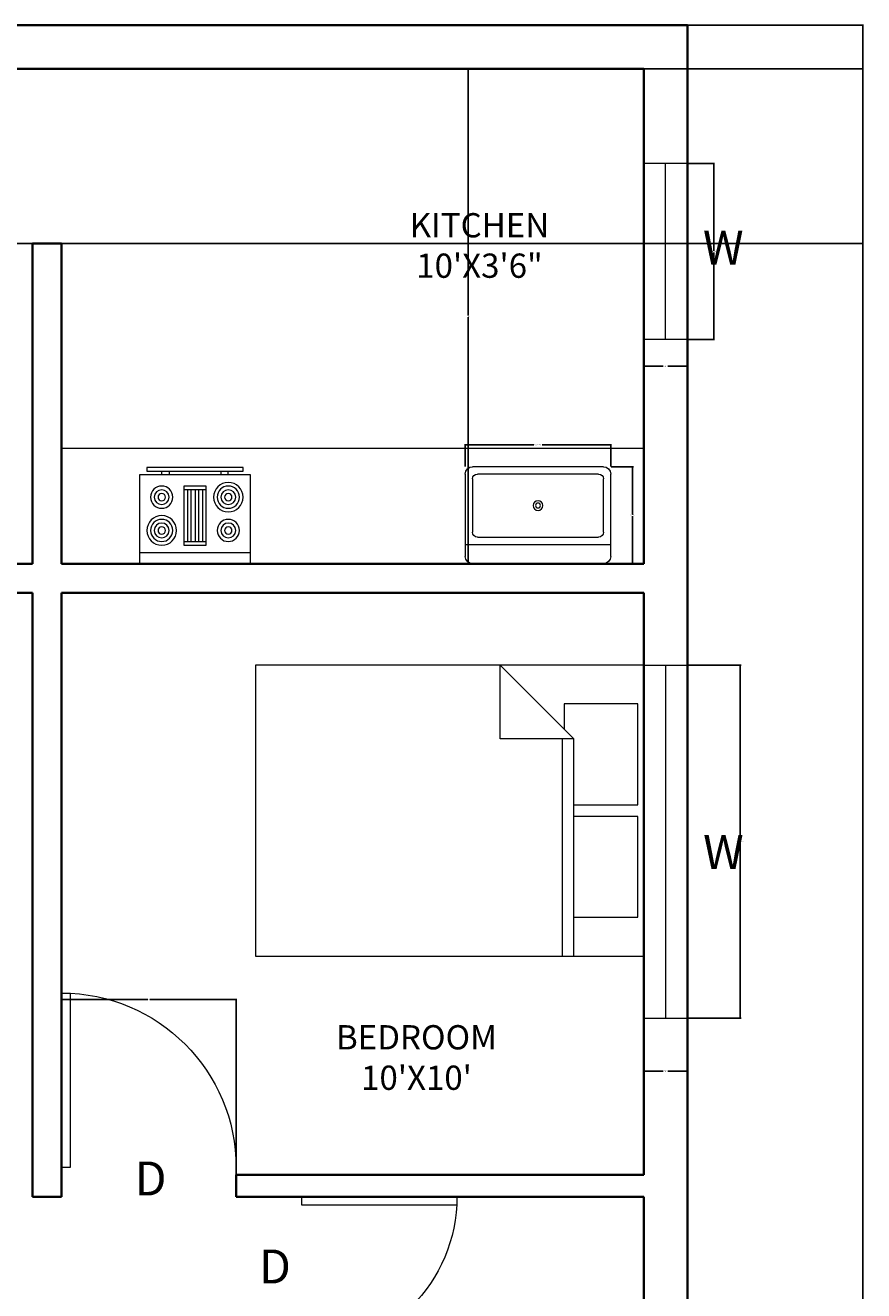
# Model space of a CAD drawing. Units: inches. Extents: x 1939 to 2674, y 558 to 1170.
# Tile 6 of 6: x 2502 to 2674, y 873 to 1134. Entities that reach past the tile are written whole.
import ezdxf

# ---------------------------------------------------------------- set-up
doc = ezdxf.new("R2010")
doc.units = ezdxf.units.IN
for name, color, linetype, lineweight in [('A-ANNO-DIMS', 2, 'Continuous', 18), ('A-ANNO-TEXT', 7, 'Continuous', 18), ('A-AREA-IDEN', 7, 'Continuous', 18), ('A-DOOR', 3, 'Continuous', 18), ('A-EQPM', 8, 'Continuous', 18), ('A-FLOR-CASE', 8, 'Continuous', 18), ('A-FLOR-FIXT', 9, 'Continuous', 18), ('A-FURN', 8, 'Continuous', 13), ('A-GLAZ', 4, 'Continuous', 18), ('A-WALL', 7, 'Continuous', 35)]:
    doc.layers.add(name, color=color, linetype=linetype, lineweight=lineweight)
doc.styles.get("Standard").update_dxf_attribs({"font": 'arial.ttf'})
doc.dimstyles.get("Standard").update_dxf_attribs({"dimtxt": 0.18, "dimasz": 0.18, "dimexe": 0.18, "dimexo": 0.0625, "dimgap": 0.09, "dimtad": 0, "dimtih": 1, "dimtoh": 1, "dimdec": 4, "dimzin": 0, "dimdsep": 46, "dimtxsty": 'Standard', "dimcen": 0.09, "dimadec": 0, "dimazin": 0, "dimtfac": 1, "dimtdec": 4, "dimtofl": 0, "dimtmove": 0, "dimatfit": 3, "dimfxl": 1, "dimtolj": 1, "dimtzin": 0, "dimarcsym": 0})

# ---------------------------------------------------------------- blocks, each defined once
blk = doc.blocks.new('Bed - Queen')
for p, q in [((0, -80.00003), (0, 0)), ((0, 0), (59.99999, 0)), ((59.99999, 0), (59.99999, -80.00003)), ((7.99999, -1.2), (28.79998, -1.2)), ((7.99999, -14.4), (7.99999, -1.2)), ((28.79998, -1.2), (28.79998, -14.4)), ((31.19999, -1.2), (51.99999, -1.2)), ((31.19999, -14.4), (31.19999, -1.2)), ((51.99999, -1.2), (51.99999, -16.4)), ((0, -14.4), (44.8, -14.4)), ((59.99999, -29.6), (44.8, -14.4)), ((44.8, -14.4), (44.8, -29.6)), ((44.8, -16.8), (0, -16.8)), ((51.99999, -16.4), (46.79936, -16.4)), ((44.8, -29.6), (59.99999, -29.6)), ((59.99999, -80.00003), (0, -80.00003))]:
    blk.add_line(p, q)
blk = doc.blocks.new('Sink-single - 30 in top')
blk.add_line((-15, -3.999996), (15, -3.999996))
for points in [[(-13.5, 0), (13.5, 0)], [(-15, -18.499996), (-15, -1.5)], [(15, -1.5), (15, -18.499996)], [(-13.5, -17.499996), (-13.5, -6.499996)], [(-12.5, -5.499996), (12.5, -5.499996)], [(13.5, -6.499996), (13.5, -17.499996)], [(13.5, -19.999996), (-13.5, -19.999996)], [(12.5, -18.499996), (-12.5, -18.499996)]]:
    blk.add_lwpolyline(points)
for radius in [1, 0.5]:
    blk.add_circle((0, -11.999996), radius)
for centre, radius, start, end in [((-13.5, -1.5), 1.5, 90, 180), ((13.5, -1.5), 1.5, 0, 90), ((-12.5, -6.499996), 1, 90, 180), ((12.5, -6.499996), 1, 0, 90), ((-12.5, -17.499996), 1, 180, 270), ((12.5, -17.499996), 1, 270, 0), ((-13.5, -18.499996), 1.5, 180, 270), ((13.5, -18.499996), 1.5, 270, 0)]:
    blk.add_arc(centre, radius, start, end)
blk = doc.blocks.new('Range-Oven - 30 in top')
for p, q in [((0, -3), (30, -3)), ((12, -6), (18, -6)), ((13, -20), (13, -6)), ((14, -6), (14, -20)), ((15, -20), (15, -6)), ((16, -6), (16, -20)), ((17, -20), (17, -6)), ((18, -20), (12, -20)), ((6, -24), (6, -25)), ((8, -25), (8, -24)), ((22, -25), (22, -24)), ((24, -24), (24, -25))]:
    blk.add_line(p, q)
for points in [[(0, -24), (0, 0), (30, 0), (30, -24)], [(12, -21), (12, -5), (18, -5), (18, -21)], [(2, -26), (2, -25), (28, -25), (28, -26)]]:
    blk.add_lwpolyline(points, close=True)
for centre, radius in [((6, -9), 4), ((6, -9), 3), ((24, -9), 3), ((6, -9), 2), ((6, -9), 1), ((24, -9), 2), ((24, -9), 1), ((6, -18), 3), ((6, -18), 2), ((6, -18), 1), ((24, -18), 4), ((24, -18), 3), ((24, -18), 2), ((24, -18), 1)]:
    blk.add_circle(centre, radius)
blk = doc.blocks.new('*U10')
for p, q in [((0, 0), (0, -6)), ((-36, 0), (-36, -6))]:
    blk.add_line(p, q)
blk.add_lwpolyline([(0, 0), (0, 36), (-1.75, 36), (-1.75, 0)], close=True)
blk.add_arc((0, 0), 36, 90, 180)
blk = doc.blocks.new('*U12')
for p, q in [((0, 0), (0, -6)), ((-32, 0), (-32, -6))]:
    blk.add_line(p, q)
blk.add_lwpolyline([(0, 0), (0, 32), (-1.75, 32), (-1.75, 0)], close=True)
blk.add_arc((0, 0), 32, 90, 180)
blk = doc.blocks.new('WIN-KITCHEN')
for p, q in [((9, 36.3), (0, 36.3)), ((4.5, 0), (4.5, 36.3)), ((9, 0), (0, 0))]:
    blk.add_line(p, q)
blk = doc.blocks.new('WIN-BEDROOM')
for p, q in [((9, 72.81), (0, 72.81)), ((4.5, 0), (4.5, 72.81)), ((9, 0), (0, 0))]:
    blk.add_line(p, q)
blk = doc.blocks.new('*D30')
at = {"layer": 'A-ANNO-DIMS', "color": 0, "lineweight": -2, "transparency": 16777216}
for p, q in [((2592.27, 1043.17), (2592.27, 1047.79)), ((2592.45, 1047.61), (2606.41, 1047.61)), ((2622.09, 1047.61), (2608.12, 1047.61)), ((2622.27, 1043.17), (2622.27, 1047.79))]:
    blk.add_line(p, q, dxfattribs=at)
at = {"layer": 'A-ANNO-DIMS', "color": 0, "transparency": 16777216}
for points in [[(2592.45, 1047.64), (2592.45, 1047.58), (2592.27, 1047.61)], [(2622.09, 1047.64), (2622.09, 1047.58), (2622.27, 1047.61)]]:
    blk.add_solid(points, dxfattribs=at)
at = {"layer": 'Defpoints', "color": 0, "transparency": 16777216}
for p in [(2622.27, 1047.61), (2592.27, 1043.11), (2622.27, 1043.11)]:
    blk.add_point(p, dxfattribs=at)
at = {"layer": 'A-ANNO-DIMS', "color": 0, "transparency": 16777216, "insert": (2607.27, 1047.61), "char_height": 0.18, "attachment_point": 5}
blk.add_mtext('\\A1;SINK 30 TYP.', dxfattribs=at)
blk = doc.blocks.new('*D31')
at = {"layer": 'A-ANNO-DIMS', "color": 0, "lineweight": -2, "transparency": 16777216}
for p, q in [((2622.33, 1043.11), (2626.95, 1043.11)), ((2626.77, 1042.93), (2626.77, 1033.29)), ((2626.77, 1023.29), (2626.77, 1032.93)), ((2622.33, 1023.11), (2626.95, 1023.11))]:
    blk.add_line(p, q, dxfattribs=at)
at = {"layer": 'A-ANNO-DIMS', "color": 0, "transparency": 16777216}
for points in [[(2626.74, 1042.93), (2626.8, 1042.93), (2626.77, 1043.11)], [(2626.74, 1023.29), (2626.8, 1023.29), (2626.77, 1023.11)]]:
    blk.add_solid(points, dxfattribs=at)
at = {"layer": 'Defpoints', "color": 0, "transparency": 16777216}
for p in [(2622.27, 1043.11), (2622.27, 1023.11), (2626.77, 1023.11)]:
    blk.add_point(p, dxfattribs=at)
at = {"layer": 'A-ANNO-DIMS', "color": 0, "transparency": 16777216, "insert": (2626.77, 1033.11), "char_height": 0.18, "attachment_point": 5}
blk.add_mtext('\\A1;20 TYP.', dxfattribs=at)
blk = doc.blocks.new('*D40')
at = {"layer": 'A-ANNO-DIMS', "color": 0, "lineweight": -2, "transparency": 16777216}
for p, q in [((2638.11, 1105.6), (2643.67, 1105.6)), ((2643.49, 1105.42), (2643.49, 1087.64)), ((2643.49, 1069.49), (2643.49, 1087.27)), ((2638.11, 1069.31), (2643.67, 1069.31))]:
    blk.add_line(p, q, dxfattribs=at)
at = {"layer": 'A-ANNO-DIMS', "color": 0, "transparency": 16777216}
for points in [[(2643.46, 1105.42), (2643.52, 1105.42), (2643.49, 1105.6)], [(2643.46, 1069.49), (2643.52, 1069.49), (2643.49, 1069.31)]]:
    blk.add_solid(points, dxfattribs=at)
at = {"layer": 'Defpoints', "color": 0, "transparency": 16777216}
for p in [(2638.05, 1105.6), (2643.49, 1105.6), (2638.05, 1069.31)]:
    blk.add_point(p, dxfattribs=at)
at = {"layer": 'A-ANNO-DIMS', "color": 0, "transparency": 16777216, "insert": (2643.49, 1087.46), "char_height": 0.18, "attachment_point": 5}
blk.add_mtext('\\A1;WDW 36 TYP.', dxfattribs=at)
blk = doc.blocks.new('*D41')
at = {"layer": 'A-ANNO-DIMS', "color": 0, "lineweight": -2, "transparency": 16777216}
for p, q in [((2629.05, 1069.25), (2629.05, 1063.68)), ((2638.05, 1069.25), (2638.05, 1063.68)), ((2629.23, 1063.86), (2633.09, 1063.86)), ((2637.87, 1063.86), (2634.01, 1063.86))]:
    blk.add_line(p, q, dxfattribs=at)
at = {"layer": 'A-ANNO-DIMS', "color": 0, "transparency": 16777216}
for points in [[(2629.23, 1063.89), (2629.23, 1063.83), (2629.05, 1063.86)], [(2637.87, 1063.89), (2637.87, 1063.83), (2638.05, 1063.86)]]:
    blk.add_solid(points, dxfattribs=at)
at = {"layer": 'Defpoints', "color": 0, "transparency": 16777216}
for p in [(2629.05, 1069.31), (2638.05, 1069.31), (2638.05, 1063.86)]:
    blk.add_point(p, dxfattribs=at)
at = {"layer": 'A-ANNO-DIMS', "color": 0, "transparency": 16777216, "insert": (2633.55, 1063.86), "char_height": 0.18, "attachment_point": 5}
blk.add_mtext('\\A1;9 TYP.', dxfattribs=at)
blk = doc.blocks.new('*D42')
at = {"layer": 'A-ANNO-DIMS', "color": 0, "lineweight": -2, "transparency": 16777216}
for p, q in [((2638.11, 1002.22), (2649.15, 1002.22)), ((2648.97, 1002.04), (2648.97, 966)), ((2648.97, 929.59), (2648.97, 965.63)), ((2638.11, 929.41), (2649.15, 929.41))]:
    blk.add_line(p, q, dxfattribs=at)
at = {"layer": 'A-ANNO-DIMS', "color": 0, "transparency": 16777216}
for points in [[(2648.94, 1002.04), (2649, 1002.04), (2648.97, 1002.22)], [(2648.94, 929.59), (2649, 929.59), (2648.97, 929.41)]]:
    blk.add_solid(points, dxfattribs=at)
at = {"layer": 'Defpoints', "color": 0, "transparency": 16777216}
for p in [(2638.05, 1002.22), (2638.05, 929.41), (2648.97, 929.41)]:
    blk.add_point(p, dxfattribs=at)
at = {"layer": 'A-ANNO-DIMS', "color": 0, "transparency": 16777216, "insert": (2648.97, 965.82), "char_height": 0.18, "attachment_point": 5}
blk.add_mtext('\\A1;WDW 73 TYP.', dxfattribs=at)
blk = doc.blocks.new('*D43')
at = {"layer": 'A-ANNO-DIMS', "color": 0, "lineweight": -2, "transparency": 16777216}
for p, q in [((2629.05, 929.35), (2629.05, 918.31)), ((2638.05, 929.35), (2638.05, 918.31)), ((2629.23, 918.49), (2633.09, 918.49)), ((2637.87, 918.49), (2634.01, 918.49))]:
    blk.add_line(p, q, dxfattribs=at)
at = {"layer": 'A-ANNO-DIMS', "color": 0, "transparency": 16777216}
for points in [[(2629.23, 918.52), (2629.23, 918.46), (2629.05, 918.49)], [(2637.87, 918.52), (2637.87, 918.46), (2638.05, 918.49)]]:
    blk.add_solid(points, dxfattribs=at)
at = {"layer": 'Defpoints', "color": 0, "transparency": 16777216}
for p in [(2629.05, 929.41), (2638.05, 929.41), (2629.05, 918.49)]:
    blk.add_point(p, dxfattribs=at)
at = {"layer": 'A-ANNO-DIMS', "color": 0, "transparency": 16777216, "insert": (2633.55, 918.49), "char_height": 0.18, "attachment_point": 5}
blk.add_mtext('\\A1;9 TYP.', dxfattribs=at)
blk = doc.blocks.new('*D50')
at = {"layer": 'A-ANNO-DIMS', "color": 0, "lineweight": -2, "transparency": 16777216}
for p, q in [((2638.11, 1134.11), (2674.38, 1134.11)), ((2674.2, 1133.93), (2674.2, 864.29)), ((2674.2, 594.29), (2674.2, 863.93)), ((2638.11, 594.11), (2674.38, 594.11))]:
    blk.add_line(p, q, dxfattribs=at)
at = {"layer": 'A-ANNO-DIMS', "color": 0, "transparency": 16777216}
for points in [[(2674.17, 1133.93), (2674.23, 1133.93), (2674.2, 1134.11)], [(2674.17, 594.29), (2674.23, 594.29), (2674.2, 594.11)]]:
    blk.add_solid(points, dxfattribs=at)
at = {"layer": 'Defpoints', "color": 0, "transparency": 16777216}
for p in [(2638.05, 1134.11), (2674.2, 1134.11), (2638.05, 594.11)]:
    blk.add_point(p, dxfattribs=at)
at = {"layer": 'A-ANNO-DIMS', "color": 0, "transparency": 16777216, "insert": (2674.2, 864.11), "char_height": 0.18, "attachment_point": 5}
blk.add_mtext('\\A1;540', dxfattribs=at)
blk = doc.blocks.new('*D54')
at = {"layer": 'A-ANNO-DIMS', "color": 0, "lineweight": -2, "transparency": 16777216}
for p, q in [((2509.05, 897.17), (2509.05, 933.44)), ((2509.23, 933.26), (2526.83, 933.26)), ((2544.87, 933.26), (2527.27, 933.26)), ((2545.05, 897.17), (2545.05, 933.44))]:
    blk.add_line(p, q, dxfattribs=at)
at = {"layer": 'A-ANNO-DIMS', "color": 0, "transparency": 16777216}
for points in [[(2509.23, 933.29), (2509.23, 933.23), (2509.05, 933.26)], [(2544.87, 933.29), (2544.87, 933.23), (2545.05, 933.26)]]:
    blk.add_solid(points, dxfattribs=at)
at = {"layer": 'Defpoints', "color": 0, "transparency": 16777216}
for p in [(2545.05, 933.26), (2509.05, 897.11), (2545.05, 897.11)]:
    blk.add_point(p, dxfattribs=at)
at = {"layer": 'A-ANNO-DIMS', "color": 0, "transparency": 16777216, "insert": (2527.05, 933.26), "char_height": 0.18, "attachment_point": 5}
blk.add_mtext('\\A1;36', dxfattribs=at)
blk = doc.blocks.new('*D65')
at = {"layer": 'A-ANNO-DIMS', "color": 0, "lineweight": -2, "transparency": 16777216}
for p, q in [((2122.29, 1125.11), (2674.38, 1125.11)), ((2674.2, 1124.93), (2674.2, 1107.29)), ((2674.2, 1089.29), (2674.2, 1106.93)), ((2104.11, 1089.11), (2674.38, 1089.11))]:
    blk.add_line(p, q, dxfattribs=at)
at = {"layer": 'A-ANNO-DIMS', "color": 0, "transparency": 16777216}
for points in [[(2674.17, 1124.93), (2674.23, 1124.93), (2674.2, 1125.11)], [(2674.17, 1089.29), (2674.23, 1089.29), (2674.2, 1089.11)]]:
    blk.add_solid(points, dxfattribs=at)
at = {"layer": 'Defpoints', "color": 0, "transparency": 16777216}
for p in [(2122.22, 1125.11), (2674.2, 1125.11), (2104.05, 1089.11)]:
    blk.add_point(p, dxfattribs=at)
at = {"layer": 'A-ANNO-DIMS', "color": 0, "transparency": 16777216, "insert": (2674.2, 1107.11), "char_height": 0.18, "attachment_point": 5}
blk.add_mtext('\\A1;36', dxfattribs=at)
blk = doc.blocks.new('*D67')
at = {"layer": 'A-ANNO-DIMS', "color": 0, "lineweight": -2, "transparency": 16777216}
for p, q in [((2628.99, 1125.11), (2592.72, 1125.11)), ((2592.9, 1124.93), (2592.9, 1074.29)), ((2592.9, 1023.29), (2592.9, 1073.93)), ((2628.99, 1023.11), (2592.72, 1023.11))]:
    blk.add_line(p, q, dxfattribs=at)
at = {"layer": 'A-ANNO-DIMS', "color": 0, "transparency": 16777216}
for points in [[(2592.87, 1124.93), (2592.93, 1124.93), (2592.9, 1125.11)], [(2592.87, 1023.29), (2592.93, 1023.29), (2592.9, 1023.11)]]:
    blk.add_solid(points, dxfattribs=at)
at = {"layer": 'Defpoints', "color": 0, "transparency": 16777216}
for p in [(2592.9, 1125.11), (2629.05, 1125.11), (2629.05, 1023.11)]:
    blk.add_point(p, dxfattribs=at)
at = {"layer": 'A-ANNO-DIMS', "color": 0, "transparency": 16777216, "insert": (2592.9, 1074.11), "char_height": 0.18, "attachment_point": 5}
blk.add_mtext('\\A1;102', dxfattribs=at)

msp = doc.modelspace()

# ---------------------------------------------------------------- linework, layer by layer
at = {"layer": 'A-FLOR-CASE'}
msp.add_line((2629.048, 1046.8584), (2509.048, 1046.8584), dxfattribs=at)
at = {"layer": 'A-WALL'}
for p, q in [((2638.048, 1134.1102), (1975.048, 1134.1102)), ((2638.048, 594.1102), (2638.048, 1134.1102)), ((2638.048, 1134.1102), (2638.048, 594.1102)), ((2629.048, 1125.1102), (2383.048, 1125.1102)), ((2629.048, 1125.1102), (2629.048, 1023.1102)), ((2503.048, 1089.1102), (2503.048, 1023.1102)), ((2509.048, 1089.1102), (2503.048, 1089.1102)), ((2509.048, 1089.1102), (2509.048, 1023.1102)), ((2483.6519, 1023.1102), (2503.048, 1023.1102)), ((2509.048, 1023.1102), (2629.048, 1023.1102)), ((2483.6519, 1017.1102), (2503.048, 1017.1102)), ((2503.048, 1017.1102), (2503.048, 892.6102)), ((2509.048, 1017.1102), (2629.048, 1017.1102)), ((2509.048, 1017.1102), (2509.048, 897.1102)), ((2629.048, 1017.1102), (2629.048, 897.1102)), ((2509.048, 897.1102), (2509.048, 892.6102)), ((2545.048, 897.1102), (2629.048, 897.1102)), ((2545.048, 897.1102), (2545.048, 892.6102)), ((2503.048, 892.6102), (2509.048, 892.6102)), ((2545.048, 892.6102), (2629.048, 892.6102)), ((2629.048, 892.6102), (2629.048, 775.6102))]:
    msp.add_line(p, q, dxfattribs=at)

# ---------------------------------------------------------------- block references
at = {"layer": 'A-DOOR', "xscale": -1}
msp.add_blockref('*U10', (2509.048, 898.6102), dxfattribs=at)
at = {"layer": 'A-DOOR', "xscale": -1, "rotation": 270}
msp.add_blockref('*U12', (2558.548, 892.6102), dxfattribs=at)
at = {"layer": 'A-EQPM', "xscale": -0.762387585591576, "yscale": 0.762387585591576, "zscale": 0.762387585591576, "rotation": 180}
msp.add_blockref('Range-Oven - 30 in top', (2525.1249, 1023.1102), dxfattribs=at)
at = {"layer": 'A-FLOR-FIXT', "xscale": -1, "rotation": 180}
msp.add_blockref('Sink-single - 30 in top', (2607.2656, 1023.1102), dxfattribs=at)
at = {"layer": 'A-FURN', "xscale": -1, "rotation": 270}
msp.add_blockref('Bed - Queen', (2629.048, 942.2222), dxfattribs=at)
at = {"layer": 'A-GLAZ'}
msp.add_blockref('WIN-KITCHEN', (2629.048, 1069.3076), dxfattribs=at)
at = {"layer": 'A-GLAZ', "rotation": 180}
msp.add_blockref('WIN-BEDROOM', (2638.048, 1002.2222), dxfattribs=at)

# ---------------------------------------------------------------- texts
at = {"layer": 'A-ANNO-TEXT', "char_height": 7, "attachment_point": 3}
for s, insert in [('\\pxqc;W', (2656.4061, 1091.745)), ('\\pxqc;W', (2656.4343, 967.1949)), ('\\pxqc;D', (2538.356, 899.8795)), ('\\pxqc;D', (2563.9822, 881.735))]:
    msp.add_mtext_dynamic_manual_height_columns(s, width=21.893501, gutter_width=12.5, heights=[0], dxfattribs=dict(at, insert=insert))
at = {"layer": 'A-AREA-IDEN', "char_height": 5, "attachment_point": 3}
for s, insert in [('\\pxqc;KITCHEN\\P10\'X3\'6"', (2614.7585, 1095.3899)), ("\\pxqc;BEDROOM\\P10'X10'", (2601.7753, 927.9875))]:
    msp.add_mtext_dynamic_manual_height_columns(s, width=39.116177, gutter_width=12.5, heights=[0], dxfattribs=dict(at, insert=insert))

# ---------------------------------------------------------------- dimensions: what is measured, and where the dimension line sits
at = {"layer": 'A-ANNO-DIMS'}
for base, p1, p2, picture, middle in [((2674.198, 1134.1102), (2638.048, 594.1102), (2638.048, 1134.1102), '*D50', (2674.198, 864.1102)), ((2674.198, 1125.1102), (2104.048, 1089.1102), (2122.2249, 1125.1102), '*D65', (2674.198, 1107.1102)), ((2592.898, 1125.1102), (2629.048, 1023.1102), (2629.048, 1125.1102), '*D67', (2592.898, 1074.1102))]:
    dim = msp.add_linear_dim(base=base, p1=p1, p2=p2, angle=90, dimstyle='Standard', override={"dimdec": 0, "dimlfac": 1, "dimrnd": 0, "dimzin": 0, "dimdsep": 46, "dimlunit": 2}, dxfattribs=at)
    dim.commit()
    dim.dimension.update_dxf_attribs({"geometry": picture, "text_midpoint": middle})
for base, p1, p2, angle, text, picture, middle in [((2643.4923, 1105.6031), (2638.048, 1069.3076), (2638.048, 1105.6031), 90, 'WDW <> TYP.', '*D40', (2643.4923, 1087.4554)), ((2626.7656, 1023.1102), (2622.2656, 1043.1102), (2622.2656, 1023.1102), 270, '<> TYP.', '*D31', (2626.7656, 1033.1102)), ((2648.9697, 929.4108), (2638.048, 1002.2222), (2638.048, 929.4108), 270, 'WDW <> TYP.', '*D42', (2648.9697, 965.8165)), ((2629.048, 918.4891), (2638.048, 929.4108), (2629.048, 929.4108), 180, '<> TYP.', '*D43', (2633.548, 918.4891))]:
    dim = msp.add_linear_dim(base=base, p1=p1, p2=p2, angle=angle, text=text, dimstyle='Standard', override={"dimdec": 0, "dimlfac": 1, "dimrnd": 0, "dimzin": 0, "dimdsep": 46, "dimlunit": 2}, dxfattribs=at)
    dim.commit()
    dim.dimension.update_dxf_attribs({"geometry": picture, "text_midpoint": middle})
for base, p1, p2, text, picture, middle in [((2638.048, 1063.8633), (2629.048, 1069.3076), (2638.048, 1069.3076), '<> TYP.', '*D41', (2633.548, 1063.8633)), ((2622.2656, 1047.6102), (2592.2656, 1043.1102), (2622.2656, 1043.1102), 'SINK <> TYP.', '*D30', (2607.2656, 1047.6102))]:
    dim = msp.add_linear_dim(base=base, p1=p1, p2=p2, text=text, dimstyle='Standard', override={"dimdec": 0, "dimlfac": 1, "dimrnd": 0, "dimzin": 0, "dimdsep": 46, "dimlunit": 2}, dxfattribs=at)
    dim.commit()
    dim.dimension.update_dxf_attribs({"geometry": picture, "text_midpoint": middle})
dim = msp.add_linear_dim(base=(2545.048, 933.2602), p1=(2509.048, 897.1102), p2=(2545.048, 897.1102), dimstyle='Standard', override={"dimdec": 0, "dimlfac": 1, "dimrnd": 0, "dimzin": 0, "dimdsep": 46, "dimlunit": 2}, dxfattribs=at)
dim.commit()
dim.dimension.update_dxf_attribs({"geometry": '*D54', "text_midpoint": (2527.048, 933.2602)})

doc.saveas('drawing.dxf')
